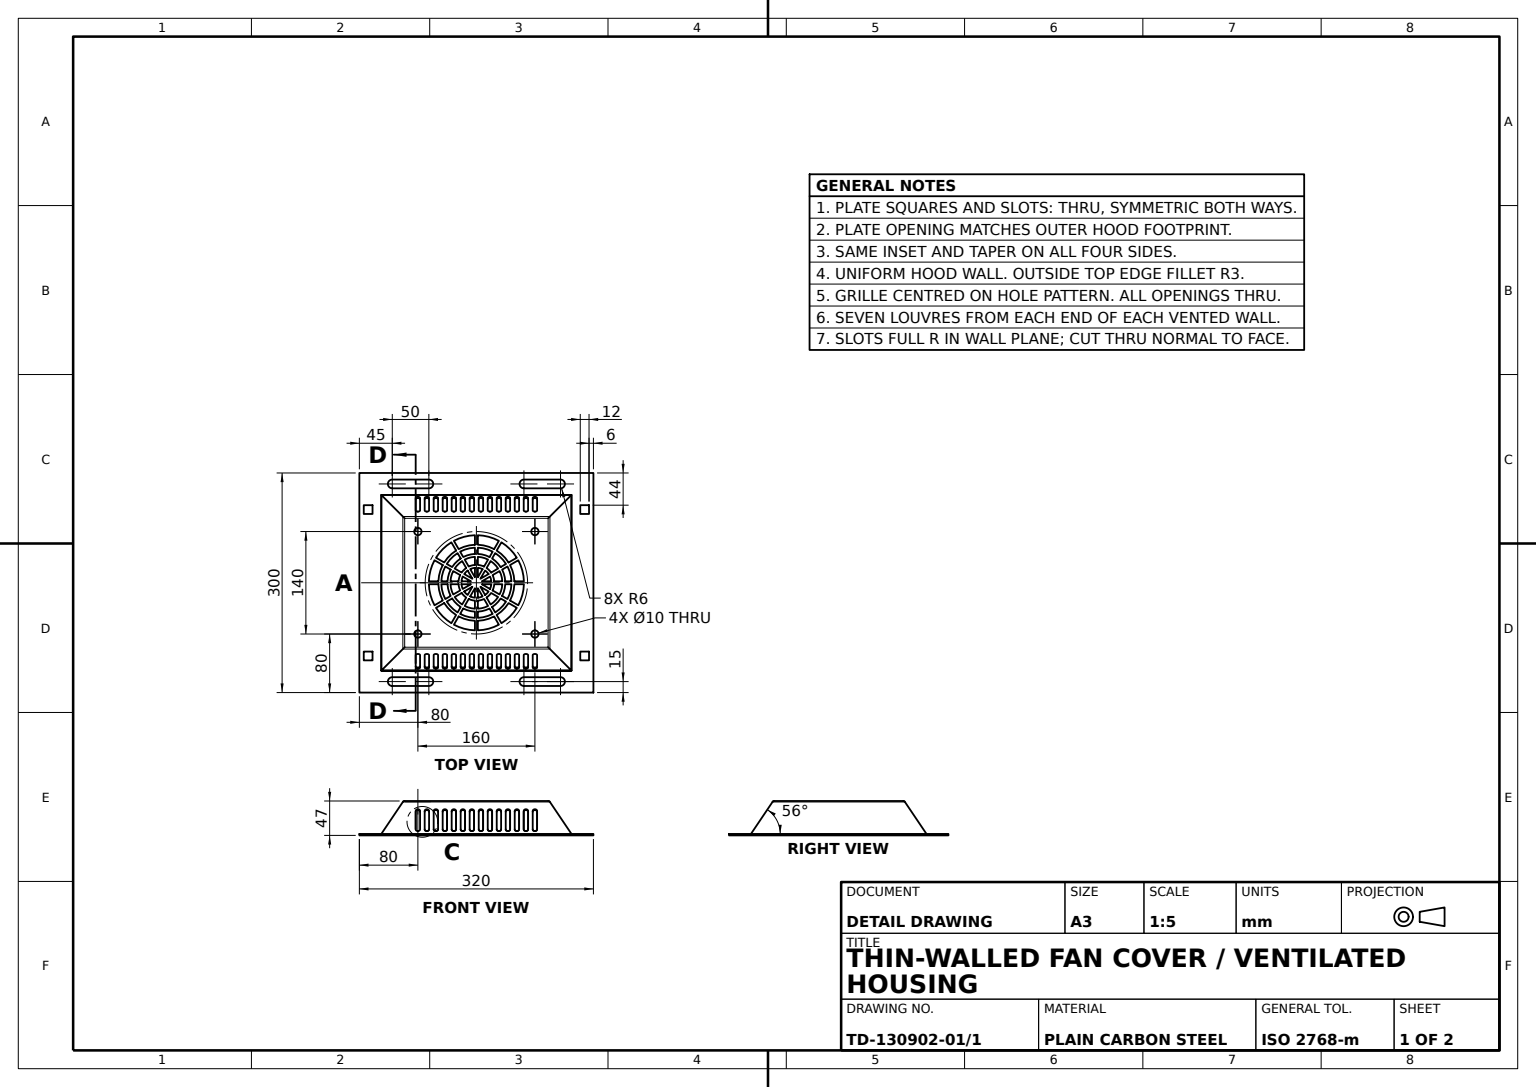
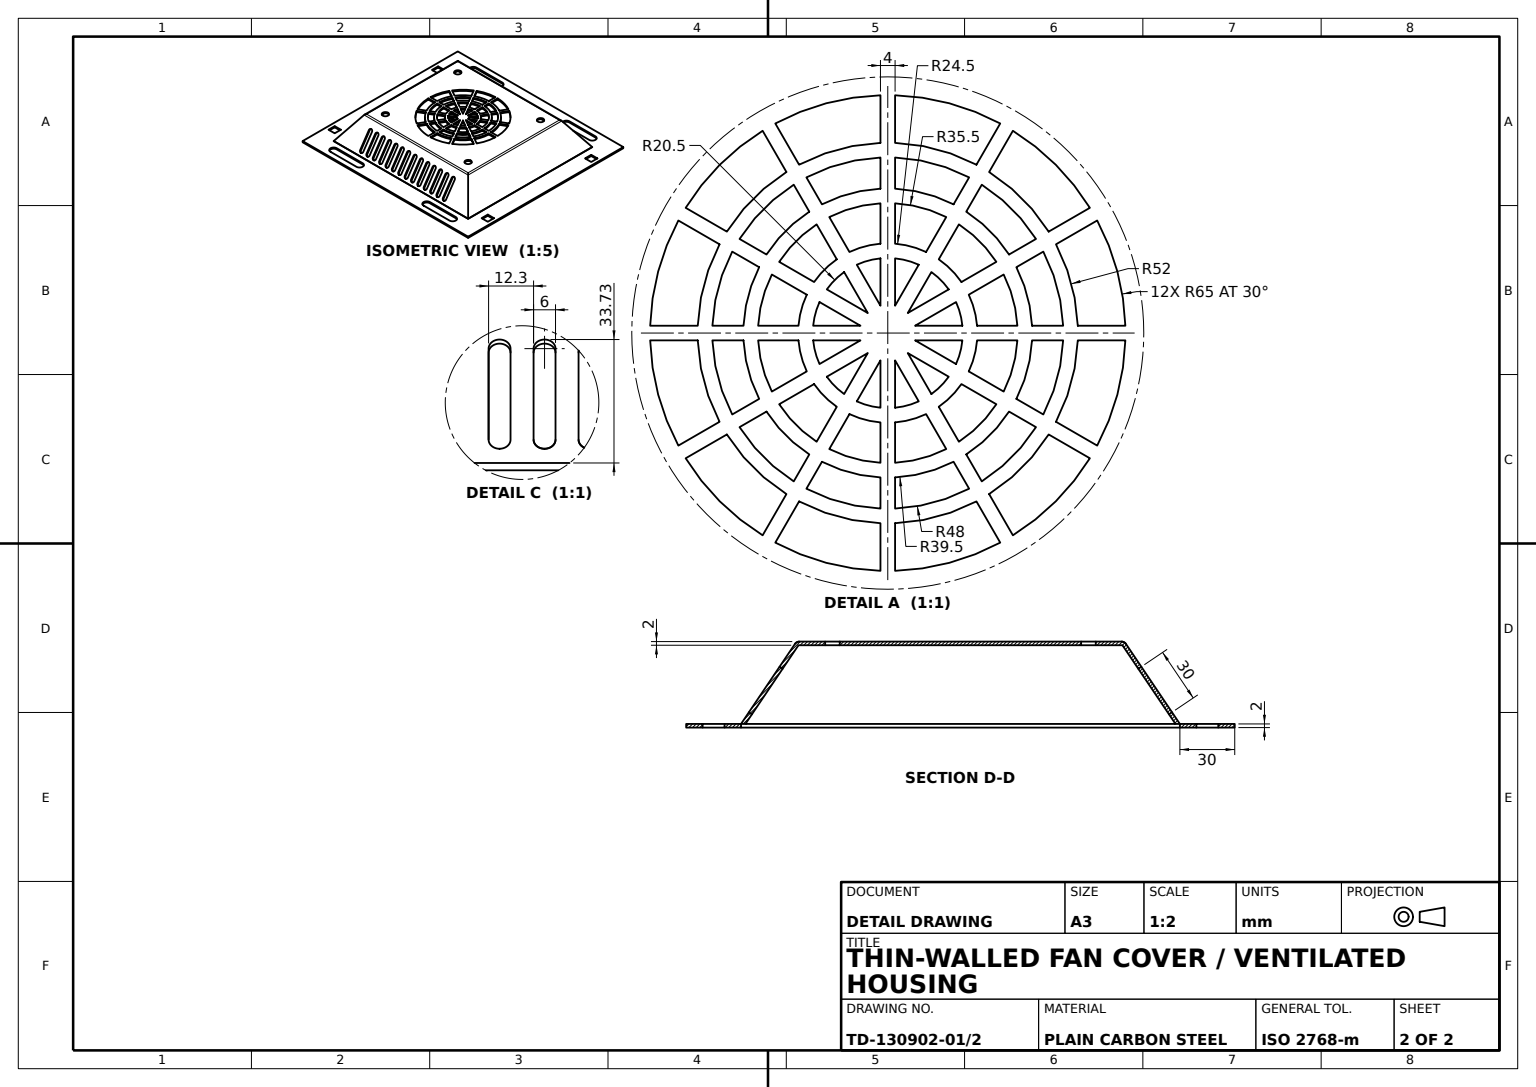
from build123d import *

# Parameters (mm, degrees)
BASE_PLATE_SKETCH_W                  = 320
BASE_PLATE_SKETCH_H                  = 300
BASE_PLATE_320X300X2_DEPTH           = 2
HOOD_FOOTPRINT_SKETCH_W              = 260
HOOD_FOOTPRINT_SKETCH_H              = 240
TAPERED_HOOD_H45_DEPTH               = 45
TAPERED_HOOD_H45_TAPER               = 34
HOOD_OPENING_SKETCH_W                = 260
HOOD_OPENING_SKETCH_H                = 240
HOOD_UNDERSIDE_OPENING_DEPTH         = 2
HOOD_SHELL_2MM_T                     = -2
FAN_GRILLE_CUT_DEPTH                 = 2
HOOD_EDGE_FILLET_R3_R                = 3
LOUVRE_SLOTS_SIDE_A_DEPTH            = 2
LOUVRE_SLOTS_SIDE_B_DEPTH            = 2
PLATE_MOUNTING_SLOTS_SKETCH_W        = 12
PLATE_MOUNTING_SLOTS_SKETCH_H        = 12
PLATE_MOUNTING_SLOTS_AND_HOLES_DEPTH = 2
HOOD_TOP_HOLES_SKETCH_R              = 5
HOOD_TOP_FIXING_HOLES_DEPTH          = 2


with BuildPart() as part:
    # Base Plate Sketch → Base Plate 320x300x2 (new body)
    with BuildSketch(Plane(origin=(0, 0, 0), x_dir=(1, 0, 0), z_dir=(0, 1, 0))):
        Rectangle(BASE_PLATE_SKETCH_W, BASE_PLATE_SKETCH_H)
    extrude(amount=BASE_PLATE_320X300X2_DEPTH)

    # Hood Footprint Sketch → Tapered Hood H45 (add)
    with BuildSketch(Plane(origin=(0, 2, 0), x_dir=(1, 0, 0), z_dir=(0, 1, 0))):
        Rectangle(HOOD_FOOTPRINT_SKETCH_W, HOOD_FOOTPRINT_SKETCH_H)
    extrude(amount=TAPERED_HOOD_H45_DEPTH, taper=TAPERED_HOOD_H45_TAPER)

    # Hood Opening Sketch → Hood Underside Opening (cut)
    with BuildSketch(Plane.XZ):
        Rectangle(HOOD_OPENING_SKETCH_W, HOOD_OPENING_SKETCH_H)
    extrude(amount=-HOOD_UNDERSIDE_OPENING_DEPTH, mode=Mode.SUBTRACT)


with BuildPart() as hood_underside_opening_piece_1:
    # of the separate pieces the step leaves, piece 1, a body of its own (hood_underside_opening_pieces)
    add(part.part.solids().sort_by_distance((99.647116742, 47, 89.647116742))[0])

    # Hood Shell 2mm
    hood_shell_2mm_openings = [hood_underside_opening_piece_1.faces().sort_by_distance(p)[0] for p in [
        (0, 2, 0),
    ]]
    offset(amount=HOOD_SHELL_2MM_T, openings=hood_shell_2mm_openings, kind=Kind.INTERSECTION)

    # Fan Grille Sketch → Fan Grille Cut (cut)
    with BuildSketch(Plane(origin=(0, 47, 0), x_dir=(1, 0, 0), z_dir=(0, 1, 0))):
        with BuildLine():
            ThreePointArc((-27.712812921, 44), (-36.769552622, 36.769552622), (-44, 27.712812921))
            Line((-44, 27.712812921), (-55.264998001, 34.216662549))
            ThreePointArc((-55.264998001, 34.216662549), (-45.961940777, 45.961940777), (-34.216662549, 55.264998001))
            Line((-34.216662549, 55.264998001), (-27.712812921, 44))
        make_face()
        with BuildLine():
            Line((-30.752560934, 57.264998001), (-24.248711306, 46))
            ThreePointArc((-24.248711306, 46), (-13.458590345, 50.228142967), (-2, 51.961524227))
            Line((-2, 51.961524227), (-2, 64.969223483))
            ThreePointArc((-2, 64.969223483), (-16.823237932, 62.785178709), (-30.752560934, 57.264998001))
        make_face()
        with BuildLine():
            ThreePointArc((30.752560934, 57.264998001), (16.823237932, 62.785178709), (2, 64.969223483))
            Line((2, 64.969223483), (2, 51.961524227))
            ThreePointArc((2, 51.961524227), (13.458590345, 50.228142967), (24.248711306, 46))
            Line((24.248711306, 46), (30.752560934, 57.264998001))
        make_face()
        with BuildLine():
            ThreePointArc((44, 27.712812921), (36.769552622, 36.769552622), (27.712812921, 44))
            Line((27.712812921, 44), (34.216662549, 55.264998001))
            ThreePointArc((34.216662549, 55.264998001), (45.961940777, 45.961940777), (55.264998001, 34.216662549))
            Line((55.264998001, 34.216662549), (44, 27.712812921))
        make_face()
        with BuildLine():
            ThreePointArc((51.961524227, 2), (50.228142967, 13.458590345), (46, 24.248711306))
            Line((46, 24.248711306), (57.264998001, 30.752560934))
            ThreePointArc((57.264998001, 30.752560934), (62.785178709, 16.823237932), (64.969223483, 2))
            Line((64.969223483, 2), (51.961524227, 2))
        make_face()
        with BuildLine():
            ThreePointArc((46, -24.248711306), (50.228142967, -13.458590345), (51.961524227, -2))
            Line((51.961524227, -2), (64.969223483, -2))
            ThreePointArc((64.969223483, -2), (62.785178709, -16.823237932), (57.264998001, -30.752560934))
            Line((57.264998001, -30.752560934), (46, -24.248711306))
        make_face()
        with BuildLine():
            ThreePointArc((27.712812921, -44), (36.769552622, -36.769552622), (44, -27.712812921))
            Line((44, -27.712812921), (55.264998001, -34.216662549))
            ThreePointArc((55.264998001, -34.216662549), (45.961940777, -45.961940777), (34.216662549, -55.264998001))
            Line((34.216662549, -55.264998001), (27.712812921, -44))
        make_face()
        with BuildLine():
            ThreePointArc((2, -51.961524227), (13.458590345, -50.228142967), (24.248711306, -46))
            Line((24.248711306, -46), (30.752560934, -57.264998001))
            ThreePointArc((30.752560934, -57.264998001), (16.823237932, -62.785178709), (2, -64.969223483))
            Line((2, -64.969223483), (2, -51.961524227))
        make_face()
        with BuildLine():
            ThreePointArc((-24.248711306, -46), (-13.458590345, -50.228142967), (-2, -51.961524227))
            Line((-2, -51.961524227), (-2, -64.969223483))
            ThreePointArc((-2, -64.969223483), (-16.823237932, -62.785178709), (-30.752560934, -57.264998001))
            Line((-30.752560934, -57.264998001), (-24.248711306, -46))
        make_face()
        with BuildLine():
            ThreePointArc((-44, -27.712812921), (-36.769552622, -36.769552622), (-27.712812921, -44))
            Line((-27.712812921, -44), (-34.216662549, -55.264998001))
            ThreePointArc((-34.216662549, -55.264998001), (-45.961940777, -45.961940777), (-55.264998001, -34.216662549))
            Line((-55.264998001, -34.216662549), (-44, -27.712812921))
        make_face()
        with BuildLine():
            ThreePointArc((-51.961524227, -2), (-50.228142967, -13.458590345), (-46, -24.248711306))
            Line((-46, -24.248711306), (-57.264998001, -30.752560934))
            ThreePointArc((-57.264998001, -30.752560934), (-62.785178709, -16.823237932), (-64.969223483, -2))
            Line((-64.969223483, -2), (-51.961524227, -2))
        make_face()
        with BuildLine():
            ThreePointArc((-46, 24.248711306), (-50.228142967, 13.458590345), (-51.961524227, 2))
            Line((-51.961524227, 2), (-64.969223483, 2))
            ThreePointArc((-64.969223483, 2), (-62.785178709, 16.823237932), (-57.264998001, 30.752560934))
            Line((-57.264998001, 30.752560934), (-46, 24.248711306))
        make_face()
        with BuildLine():
            ThreePointArc((-35.164125922, 17.99261649), (-38.154070138, 10.223352282), (-39.449334595, 2))
            Line((-39.449334595, 2), (-47.958315233, 2))
            ThreePointArc((-47.958315233, 2), (-46.364439662, 12.423314165), (-42.533119315, 22.247106809))
            Line((-42.533119315, 22.247106809), (-35.164125922, 17.99261649))
        make_face()
        with BuildLine():
            ThreePointArc((-21.456718105, 33.164125922), (-27.930717857, 27.930717857), (-33.164125922, 21.456718105))
            Line((-33.164125922, 21.456718105), (-40.533119315, 25.711208424))
            ThreePointArc((-40.533119315, 25.711208424), (-33.941125497, 33.941125497), (-25.711208424, 40.533119315))
            Line((-25.711208424, 40.533119315), (-21.456718105, 33.164125922))
        make_face()
        with BuildLine():
            ThreePointArc((-2, 39.449334595), (-10.223352282, 38.154070138), (-17.99261649, 35.164125922))
            Line((-17.99261649, 35.164125922), (-22.247106809, 42.533119315))
            ThreePointArc((-22.247106809, 42.533119315), (-12.423314165, 46.364439662), (-2, 47.958315233))
            Line((-2, 47.958315233), (-2, 39.449334595))
        make_face()
        with BuildLine():
            ThreePointArc((17.99261649, 35.164125922), (10.223352282, 38.154070138), (2, 39.449334595))
            Line((2, 39.449334595), (2, 47.958315233))
            ThreePointArc((2, 47.958315233), (12.423314165, 46.364439662), (22.247106809, 42.533119315))
            Line((22.247106809, 42.533119315), (17.99261649, 35.164125922))
        make_face()
        with BuildLine():
            ThreePointArc((33.164125922, 21.456718105), (27.930717857, 27.930717857), (21.456718105, 33.164125922))
            Line((21.456718105, 33.164125922), (25.711208424, 40.533119315))
            ThreePointArc((25.711208424, 40.533119315), (33.941125497, 33.941125497), (40.533119315, 25.711208424))
            Line((40.533119315, 25.711208424), (33.164125922, 21.456718105))
        make_face()
        with BuildLine():
            ThreePointArc((39.449334595, 2), (38.154070138, 10.223352282), (35.164125922, 17.99261649))
            Line((35.164125922, 17.99261649), (42.533119315, 22.247106809))
            ThreePointArc((42.533119315, 22.247106809), (46.364439662, 12.423314165), (47.958315233, 2))
            Line((47.958315233, 2), (39.449334595, 2))
        make_face()
        with BuildLine():
            ThreePointArc((35.164125922, -17.99261649), (38.154070138, -10.223352282), (39.449334595, -2))
            Line((39.449334595, -2), (47.958315233, -2))
            ThreePointArc((47.958315233, -2), (46.364439662, -12.423314165), (42.533119315, -22.247106809))
            Line((42.533119315, -22.247106809), (35.164125922, -17.99261649))
        make_face()
        with BuildLine():
            ThreePointArc((21.456718105, -33.164125922), (27.930717857, -27.930717857), (33.164125922, -21.456718105))
            Line((33.164125922, -21.456718105), (40.533119315, -25.711208424))
            ThreePointArc((40.533119315, -25.711208424), (33.941125497, -33.941125497), (25.711208424, -40.533119315))
            Line((25.711208424, -40.533119315), (21.456718105, -33.164125922))
        make_face()
        with BuildLine():
            ThreePointArc((2, -39.449334595), (10.223352282, -38.154070138), (17.99261649, -35.164125922))
            Line((17.99261649, -35.164125922), (22.247106809, -42.533119315))
            ThreePointArc((22.247106809, -42.533119315), (12.423314165, -46.364439662), (2, -47.958315233))
            Line((2, -47.958315233), (2, -39.449334595))
        make_face()
        with BuildLine():
            ThreePointArc((-17.99261649, -35.164125922), (-10.223352282, -38.154070138), (-2, -39.449334595))
            Line((-2, -39.449334595), (-2, -47.958315233))
            ThreePointArc((-2, -47.958315233), (-12.423314165, -46.364439662), (-22.247106809, -42.533119315))
            Line((-22.247106809, -42.533119315), (-17.99261649, -35.164125922))
        make_face()
        with BuildLine():
            ThreePointArc((-33.164125922, -21.456718105), (-27.930717857, -27.930717857), (-21.456718105, -33.164125922))
            Line((-21.456718105, -33.164125922), (-25.711208424, -40.533119315))
            ThreePointArc((-25.711208424, -40.533119315), (-33.941125497, -33.941125497), (-40.533119315, -25.711208424))
            Line((-40.533119315, -25.711208424), (-33.164125922, -21.456718105))
        make_face()
        with BuildLine():
            ThreePointArc((-39.449334595, -2), (-38.154070138, -10.223352282), (-35.164125922, -17.99261649))
            Line((-35.164125922, -17.99261649), (-42.533119315, -22.247106809))
            ThreePointArc((-42.533119315, -22.247106809), (-46.364439662, -12.423314165), (-47.958315233, -2))
            Line((-47.958315233, -2), (-39.449334595, -2))
        make_face()
        with BuildLine():
            ThreePointArc((-10.47706464, -22.14680827), (-6.341066605, -23.665182744), (-2, -24.418230894))
            Line((-2, -24.418230894), (-2, -35.443617197))
            ThreePointArc((-2, -35.443617197), (-9.188076101, -34.290366833), (-15.989757791, -31.695072895))
            Line((-15.989757791, -31.695072895), (-10.47706464, -22.14680827))
        make_face()
        with BuildLine():
            ThreePointArc((-20.14680827, -13.941166255), (-17.324116139, -17.324116139), (-13.941166255, -20.14680827))
            Line((-13.941166255, -20.14680827), (-19.453859406, -29.695072895))
            ThreePointArc((-19.453859406, -29.695072895), (-25.102290732, -25.102290732), (-29.695072895, -19.453859406))
            Line((-29.695072895, -19.453859406), (-20.14680827, -13.941166255))
        make_face()
        with BuildLine():
            ThreePointArc((-24.418230894, -2), (-23.665182744, -6.341066605), (-22.14680827, -10.47706464))
            Line((-22.14680827, -10.47706464), (-31.695072895, -15.989757791))
            ThreePointArc((-31.695072895, -15.989757791), (-34.290366833, -9.188076101), (-35.443617197, -2))
            Line((-35.443617197, -2), (-24.418230894, -2))
        make_face()
        with BuildLine():
            ThreePointArc((-22.14680827, 10.47706464), (-23.665182744, 6.341066605), (-24.418230894, 2))
            Line((-24.418230894, 2), (-35.443617197, 2))
            ThreePointArc((-35.443617197, 2), (-34.290366833, 9.188076101), (-31.695072895, 15.989757791))
            Line((-31.695072895, 15.989757791), (-22.14680827, 10.47706464))
        make_face()
        with BuildLine():
            ThreePointArc((-13.941166255, 20.14680827), (-17.324116139, 17.324116139), (-20.14680827, 13.941166255))
            Line((-20.14680827, 13.941166255), (-29.695072895, 19.453859406))
            ThreePointArc((-29.695072895, 19.453859406), (-25.102290732, 25.102290732), (-19.453859406, 29.695072895))
            Line((-19.453859406, 29.695072895), (-13.941166255, 20.14680827))
        make_face()
        with BuildLine():
            ThreePointArc((-2, 24.418230894), (-6.341066605, 23.665182744), (-10.47706464, 22.14680827))
            Line((-10.47706464, 22.14680827), (-15.989757791, 31.695072895))
            ThreePointArc((-15.989757791, 31.695072895), (-9.188076101, 34.290366833), (-2, 35.443617197))
            Line((-2, 35.443617197), (-2, 24.418230894))
        make_face()
        with BuildLine():
            ThreePointArc((10.47706464, 22.14680827), (6.341066605, 23.665182744), (2, 24.418230894))
            Line((2, 24.418230894), (2, 35.443617197))
            ThreePointArc((2, 35.443617197), (9.188076101, 34.290366833), (15.989757791, 31.695072895))
            Line((15.989757791, 31.695072895), (10.47706464, 22.14680827))
        make_face()
        with BuildLine():
            ThreePointArc((20.14680827, 13.941166255), (17.324116139, 17.324116139), (13.941166255, 20.14680827))
            Line((13.941166255, 20.14680827), (19.453859406, 29.695072895))
            ThreePointArc((19.453859406, 29.695072895), (25.102290732, 25.102290732), (29.695072895, 19.453859406))
            Line((29.695072895, 19.453859406), (20.14680827, 13.941166255))
        make_face()
        with BuildLine():
            ThreePointArc((24.418230894, 2), (23.665182744, 6.341066605), (22.14680827, 10.47706464))
            Line((22.14680827, 10.47706464), (31.695072895, 15.989757791))
            ThreePointArc((31.695072895, 15.989757791), (34.290366833, 9.188076101), (35.443617197, 2))
            Line((35.443617197, 2), (24.418230894, 2))
        make_face()
        with BuildLine():
            ThreePointArc((22.14680827, -10.47706464), (23.665182744, -6.341066605), (24.418230894, -2))
            Line((24.418230894, -2), (35.443617197, -2))
            ThreePointArc((35.443617197, -2), (34.290366833, -9.188076101), (31.695072895, -15.989757791))
            Line((31.695072895, -15.989757791), (22.14680827, -10.47706464))
        make_face()
        with BuildLine():
            ThreePointArc((13.941166255, -20.14680827), (17.324116139, -17.324116139), (20.14680827, -13.941166255))
            Line((20.14680827, -13.941166255), (29.695072895, -19.453859406))
            ThreePointArc((29.695072895, -19.453859406), (25.102290732, -25.102290732), (19.453859406, -29.695072895))
            Line((19.453859406, -29.695072895), (13.941166255, -20.14680827))
        make_face()
        with BuildLine():
            ThreePointArc((2, -24.418230894), (6.341066605, -23.665182744), (10.47706464, -22.14680827))
            Line((10.47706464, -22.14680827), (15.989757791, -31.695072895))
            ThreePointArc((15.989757791, -31.695072895), (9.188076101, -34.290366833), (2, -35.443617197))
            Line((2, -35.443617197), (2, -24.418230894))
        make_face()
        with BuildLine():
            Line((2, 7.464101615), (8.469052074, 18.668828484))
            ThreePointArc((8.469052074, 18.668828484), (5.305790425, 19.801479439), (2, 20.402205763))
            Line((2, 20.402205763), (2, 7.464101615))
        make_face()
        with BuildLine():
            Line((5.464101615, 5.464101615), (16.668828484, 11.933153689))
            ThreePointArc((16.668828484, 11.933153689), (14.495689014, 14.495689014), (11.933153689, 16.668828484))
            Line((11.933153689, 16.668828484), (5.464101615, 5.464101615))
        make_face()
        with BuildLine():
            Line((7.464101615, 2), (20.402205763, 2))
            ThreePointArc((20.402205763, 2), (19.801479439, 5.305790425), (18.668828484, 8.469052074))
            Line((18.668828484, 8.469052074), (7.464101615, 2))
        make_face()
        with BuildLine():
            Line((7.464101615, -2), (18.668828484, -8.469052074))
            ThreePointArc((18.668828484, -8.469052074), (19.801479439, -5.305790425), (20.402205763, -2))
            Line((20.402205763, -2), (7.464101615, -2))
        make_face()
        with BuildLine():
            Line((5.464101615, -5.464101615), (11.933153689, -16.668828484))
            ThreePointArc((11.933153689, -16.668828484), (14.495689014, -14.495689014), (16.668828484, -11.933153689))
            Line((16.668828484, -11.933153689), (5.464101615, -5.464101615))
        make_face()
        with BuildLine():
            Line((2, -20.402205763), (2, -7.464101615))
            Line((2, -7.464101615), (8.469052074, -18.668828484))
            ThreePointArc((8.469052074, -18.668828484), (5.305790425, -19.801479439), (2, -20.402205763))
        make_face()
        with BuildLine():
            Line((-2, -7.464101615), (-8.469052074, -18.668828484))
            ThreePointArc((-8.469052074, -18.668828484), (-5.305790425, -19.801479439), (-2, -20.402205763))
            Line((-2, -20.402205763), (-2, -7.464101615))
        make_face()
        with BuildLine():
            Line((-5.464101615, -5.464101615), (-16.668828484, -11.933153689))
            ThreePointArc((-16.668828484, -11.933153689), (-14.495689014, -14.495689014), (-11.933153689, -16.668828484))
            Line((-11.933153689, -16.668828484), (-5.464101615, -5.464101615))
        make_face()
        with BuildLine():
            Line((-20.402205763, -2), (-7.464101615, -2))
            Line((-7.464101615, -2), (-18.668828484, -8.469052074))
            ThreePointArc((-18.668828484, -8.469052074), (-19.801479439, -5.305790425), (-20.402205763, -2))
        make_face()
        with BuildLine():
            Line((-7.464101615, 2), (-18.668828484, 8.469052074))
            ThreePointArc((-18.668828484, 8.469052074), (-19.801479439, 5.305790425), (-20.402205763, 2))
            Line((-20.402205763, 2), (-7.464101615, 2))
        make_face()
        with BuildLine():
            Line((-5.464101615, 5.464101615), (-11.933153689, 16.668828484))
            ThreePointArc((-11.933153689, 16.668828484), (-14.495689014, 14.495689014), (-16.668828484, 11.933153689))
            Line((-16.668828484, 11.933153689), (-5.464101615, 5.464101615))
        make_face()
        with BuildLine():
            Line((-2, 7.464101615), (-2, 20.402205763))
            ThreePointArc((-2, 20.402205763), (-5.305790425, 19.801479439), (-8.469052074, 18.668828484))
            Line((-8.469052074, 18.668828484), (-2, 7.464101615))
        make_face()
    extrude(amount=-FAN_GRILLE_CUT_DEPTH, mode=Mode.SUBTRACT)

    # Hood Edge Fillet R3
    hood_edge_fillet_r3_edges = [hood_underside_opening_piece_1.edges().sort_by_distance(p)[0] for p in [
        (99.647116742, 47, 0),
        (0, 47, -89.647116742),
        (-99.647116742, 47, 0),
        (0, 47, 89.647116742),
    ]]
    fillet(hood_edge_fillet_r3_edges, radius=HOOD_EDGE_FILLET_R3_R)

    # Louvre Slots Side A Sketch → Louvre Slots Side A (cut)
    with BuildSketch(Plane(origin=(0, 56.256424681, 83.40357946), x_dir=(1, 0, 0), z_dir=(0, 0.5591929034707479, 0.829037572555041))):
        with BuildLine():
            Line((-77, -27.760393884), (-77, -57.760393884))
            ThreePointArc((-77, -57.760393884), (-80, -60.760393884), (-83, -57.760393884))
            Line((-83, -57.760393884), (-83, -27.760393884))
            ThreePointArc((-83, -27.760393884), (-80, -24.760393884), (-77, -27.760393884))
        make_face()
        with BuildLine():
            Line((83, -27.760393884), (83, -57.760393884))
            ThreePointArc((83, -57.760393884), (80, -60.760393884), (77, -57.760393884))
            Line((77, -57.760393884), (77, -27.760393884))
            ThreePointArc((77, -27.760393884), (80, -24.760393884), (83, -27.760393884))
        make_face()
        with BuildLine():
            Line((70.7, -27.760393884), (70.7, -57.760393884))
            ThreePointArc((70.7, -57.760393884), (67.7, -60.760393884), (64.7, -57.760393884))
            Line((64.7, -57.760393884), (64.7, -27.760393884))
            ThreePointArc((64.7, -27.760393884), (67.7, -24.760393884), (70.7, -27.760393884))
        make_face()
        with BuildLine():
            Line((58.4, -27.760393884), (58.4, -57.760393884))
            ThreePointArc((58.4, -57.760393884), (55.4, -60.760393884), (52.4, -57.760393884))
            Line((52.4, -57.760393884), (52.4, -27.760393884))
            ThreePointArc((52.4, -27.760393884), (55.4, -24.760393884), (58.4, -27.760393884))
        make_face()
        with BuildLine():
            Line((46.1, -27.760393884), (46.1, -57.760393884))
            ThreePointArc((46.1, -57.760393884), (43.1, -60.760393884), (40.1, -57.760393884))
            Line((40.1, -57.760393884), (40.1, -27.760393884))
            ThreePointArc((40.1, -27.760393884), (43.1, -24.760393884), (46.1, -27.760393884))
        make_face()
        with BuildLine():
            Line((33.8, -27.760393884), (33.8, -57.760393884))
            ThreePointArc((33.8, -57.760393884), (30.8, -60.760393884), (27.8, -57.760393884))
            Line((27.8, -57.760393884), (27.8, -27.760393884))
            ThreePointArc((27.8, -27.760393884), (30.8, -24.760393884), (33.8, -27.760393884))
        make_face()
        with BuildLine():
            Line((21.5, -27.760393884), (21.5, -57.760393884))
            ThreePointArc((21.5, -57.760393884), (18.5, -60.760393884), (15.5, -57.760393884))
            Line((15.5, -57.760393884), (15.5, -27.760393884))
            ThreePointArc((15.5, -27.760393884), (18.5, -24.760393884), (21.5, -27.760393884))
        make_face()
        with BuildLine():
            Line((9.2, -27.760393884), (9.2, -57.760393884))
            ThreePointArc((9.2, -57.760393884), (6.2, -60.760393884), (3.2, -57.760393884))
            Line((3.2, -57.760393884), (3.2, -27.760393884))
            ThreePointArc((3.2, -27.760393884), (6.2, -24.760393884), (9.2, -27.760393884))
        make_face()
        with BuildLine():
            Line((-64.7, -27.760393884), (-64.7, -57.760393884))
            ThreePointArc((-64.7, -57.760393884), (-67.7, -60.760393884), (-70.7, -57.760393884))
            Line((-70.7, -57.760393884), (-70.7, -27.760393884))
            ThreePointArc((-70.7, -27.760393884), (-67.7, -24.760393884), (-64.7, -27.760393884))
        make_face()
        with BuildLine():
            Line((-52.4, -27.760393884), (-52.4, -57.760393884))
            ThreePointArc((-52.4, -57.760393884), (-55.4, -60.760393884), (-58.4, -57.760393884))
            Line((-58.4, -57.760393884), (-58.4, -27.760393884))
            ThreePointArc((-58.4, -27.760393884), (-55.4, -24.760393884), (-52.4, -27.760393884))
        make_face()
        with BuildLine():
            Line((-40.1, -27.760393884), (-40.1, -57.760393884))
            ThreePointArc((-40.1, -57.760393884), (-43.1, -60.760393884), (-46.1, -57.760393884))
            Line((-46.1, -57.760393884), (-46.1, -27.760393884))
            ThreePointArc((-46.1, -27.760393884), (-43.1, -24.760393884), (-40.1, -27.760393884))
        make_face()
        with BuildLine():
            Line((-27.8, -27.760393884), (-27.8, -57.760393884))
            ThreePointArc((-27.8, -57.760393884), (-30.8, -60.760393884), (-33.8, -57.760393884))
            Line((-33.8, -57.760393884), (-33.8, -27.760393884))
            ThreePointArc((-33.8, -27.760393884), (-30.8, -24.760393884), (-27.8, -27.760393884))
        make_face()
        with BuildLine():
            Line((-15.5, -27.760393884), (-15.5, -57.760393884))
            ThreePointArc((-15.5, -57.760393884), (-18.5, -60.760393884), (-21.5, -57.760393884))
            Line((-21.5, -57.760393884), (-21.5, -27.760393884))
            ThreePointArc((-21.5, -27.760393884), (-18.5, -24.760393884), (-15.5, -27.760393884))
        make_face()
        with BuildLine():
            Line((-3.2, -27.760393884), (-3.2, -57.760393884))
            ThreePointArc((-3.2, -57.760393884), (-6.2, -60.760393884), (-9.2, -57.760393884))
            Line((-9.2, -57.760393884), (-9.2, -27.760393884))
            ThreePointArc((-9.2, -27.760393884), (-6.2, -24.760393884), (-3.2, -27.760393884))
        make_face()
    extrude(amount=-LOUVRE_SLOTS_SIDE_A_DEPTH, mode=Mode.SUBTRACT)

    # Louvre Slots Side B Sketch → Louvre Slots Side B (cut)
    with BuildSketch(Plane(origin=(0, 56.256424681, -83.40357946), x_dir=(-1, 0, 0), z_dir=(0, 0.5591929034707479, -0.829037572555041))):
        with BuildLine():
            Line((-77, -27.760393884), (-77, -57.760393884))
            ThreePointArc((-77, -57.760393884), (-80, -60.760393884), (-83, -57.760393884))
            Line((-83, -57.760393884), (-83, -27.760393884))
            ThreePointArc((-83, -27.760393884), (-80, -24.760393884), (-77, -27.760393884))
        make_face()
        with BuildLine():
            Line((83, -27.760393884), (83, -57.760393884))
            ThreePointArc((83, -57.760393884), (80, -60.760393884), (77, -57.760393884))
            Line((77, -57.760393884), (77, -27.760393884))
            ThreePointArc((77, -27.760393884), (80, -24.760393884), (83, -27.760393884))
        make_face()
        with BuildLine():
            Line((70.7, -27.760393884), (70.7, -57.760393884))
            ThreePointArc((70.7, -57.760393884), (67.7, -60.760393884), (64.7, -57.760393884))
            Line((64.7, -57.760393884), (64.7, -27.760393884))
            ThreePointArc((64.7, -27.760393884), (67.7, -24.760393884), (70.7, -27.760393884))
        make_face()
        with BuildLine():
            Line((58.4, -27.760393884), (58.4, -57.760393884))
            ThreePointArc((58.4, -57.760393884), (55.4, -60.760393884), (52.4, -57.760393884))
            Line((52.4, -57.760393884), (52.4, -27.760393884))
            ThreePointArc((52.4, -27.760393884), (55.4, -24.760393884), (58.4, -27.760393884))
        make_face()
        with BuildLine():
            Line((46.1, -27.760393884), (46.1, -57.760393884))
            ThreePointArc((46.1, -57.760393884), (43.1, -60.760393884), (40.1, -57.760393884))
            Line((40.1, -57.760393884), (40.1, -27.760393884))
            ThreePointArc((40.1, -27.760393884), (43.1, -24.760393884), (46.1, -27.760393884))
        make_face()
        with BuildLine():
            Line((33.8, -27.760393884), (33.8, -57.760393884))
            ThreePointArc((33.8, -57.760393884), (30.8, -60.760393884), (27.8, -57.760393884))
            Line((27.8, -57.760393884), (27.8, -27.760393884))
            ThreePointArc((27.8, -27.760393884), (30.8, -24.760393884), (33.8, -27.760393884))
        make_face()
        with BuildLine():
            Line((21.5, -27.760393884), (21.5, -57.760393884))
            ThreePointArc((21.5, -57.760393884), (18.5, -60.760393884), (15.5, -57.760393884))
            Line((15.5, -57.760393884), (15.5, -27.760393884))
            ThreePointArc((15.5, -27.760393884), (18.5, -24.760393884), (21.5, -27.760393884))
        make_face()
        with BuildLine():
            Line((9.2, -27.760393884), (9.2, -57.760393884))
            ThreePointArc((9.2, -57.760393884), (6.2, -60.760393884), (3.2, -57.760393884))
            Line((3.2, -57.760393884), (3.2, -27.760393884))
            ThreePointArc((3.2, -27.760393884), (6.2, -24.760393884), (9.2, -27.760393884))
        make_face()
        with BuildLine():
            Line((-64.7, -27.760393884), (-64.7, -57.760393884))
            ThreePointArc((-64.7, -57.760393884), (-67.7, -60.760393884), (-70.7, -57.760393884))
            Line((-70.7, -57.760393884), (-70.7, -27.760393884))
            ThreePointArc((-70.7, -27.760393884), (-67.7, -24.760393884), (-64.7, -27.760393884))
        make_face()
        with BuildLine():
            Line((-52.4, -27.760393884), (-52.4, -57.760393884))
            ThreePointArc((-52.4, -57.760393884), (-55.4, -60.760393884), (-58.4, -57.760393884))
            Line((-58.4, -57.760393884), (-58.4, -27.760393884))
            ThreePointArc((-58.4, -27.760393884), (-55.4, -24.760393884), (-52.4, -27.760393884))
        make_face()
        with BuildLine():
            Line((-40.1, -27.760393884), (-40.1, -57.760393884))
            ThreePointArc((-40.1, -57.760393884), (-43.1, -60.760393884), (-46.1, -57.760393884))
            Line((-46.1, -57.760393884), (-46.1, -27.760393884))
            ThreePointArc((-46.1, -27.760393884), (-43.1, -24.760393884), (-40.1, -27.760393884))
        make_face()
        with BuildLine():
            Line((-27.8, -27.760393884), (-27.8, -57.760393884))
            ThreePointArc((-27.8, -57.760393884), (-30.8, -60.760393884), (-33.8, -57.760393884))
            Line((-33.8, -57.760393884), (-33.8, -27.760393884))
            ThreePointArc((-33.8, -27.760393884), (-30.8, -24.760393884), (-27.8, -27.760393884))
        make_face()
        with BuildLine():
            Line((-15.5, -27.760393884), (-15.5, -57.760393884))
            ThreePointArc((-15.5, -57.760393884), (-18.5, -60.760393884), (-21.5, -57.760393884))
            Line((-21.5, -57.760393884), (-21.5, -27.760393884))
            ThreePointArc((-21.5, -27.760393884), (-18.5, -24.760393884), (-15.5, -27.760393884))
        make_face()
        with BuildLine():
            Line((-3.2, -27.760393884), (-3.2, -57.760393884))
            ThreePointArc((-3.2, -57.760393884), (-6.2, -60.760393884), (-9.2, -57.760393884))
            Line((-9.2, -57.760393884), (-9.2, -27.760393884))
            ThreePointArc((-9.2, -27.760393884), (-6.2, -24.760393884), (-3.2, -27.760393884))
        make_face()
    extrude(amount=-LOUVRE_SLOTS_SIDE_B_DEPTH, mode=Mode.SUBTRACT)

    # Hood Top Holes Sketch → Hood Top Fixing Holes (cut)
    with BuildSketch(Plane(origin=(0, 47, 0), x_dir=(1, 0, 0), z_dir=(0, 1, 0))):
        with Locations(Location((-80, 70, 0), (0, 0, 270))):
            Circle(HOOD_TOP_HOLES_SKETCH_R)
        with Locations(Location((80, 70, 0), (0, 0, 270))):
            Circle(HOOD_TOP_HOLES_SKETCH_R)
        with Locations(Location((80, -70, 0), (0, 0, 270))):
            Circle(HOOD_TOP_HOLES_SKETCH_R)
        with Locations(Location((-80, -70, 0), (0, 0, 270))):
            Circle(HOOD_TOP_HOLES_SKETCH_R)
    extrude(amount=-HOOD_TOP_FIXING_HOLES_DEPTH, mode=Mode.SUBTRACT)


with BuildPart() as hood_underside_opening_piece_2:
    # of the separate pieces the step leaves, piece 2, a body of its own (hood_underside_opening_pieces)
    add(part.part.solids().sort_by_distance((-160, 0, 150))[0])

    # Plate Mounting Slots Sketch → Plate Mounting Slots and Holes (cut)
    with BuildSketch(Plane(origin=(0, 2, 0), x_dir=(1, 0, 0), z_dir=(0, 1, 0))):
        with BuildLine():
            Line((-115, -129), (-65, -129))
            ThreePointArc((-65, -129), (-59, -135), (-65, -141))
            Line((-65, -141), (-115, -141))
            ThreePointArc((-115, -141), (-121, -135), (-115, -129))
        make_face()
        with BuildLine():
            Line((65, -129), (115, -129))
            ThreePointArc((115, -129), (121, -135), (115, -141))
            Line((115, -141), (65, -141))
            ThreePointArc((65, -141), (59, -135), (65, -129))
        make_face()
        with BuildLine():
            Line((-115, 141), (-65, 141))
            ThreePointArc((-65, 141), (-59, 135), (-65, 129))
            Line((-65, 129), (-115, 129))
            ThreePointArc((-115, 129), (-121, 135), (-115, 141))
        make_face()
        with BuildLine():
            Line((65, 141), (115, 141))
            ThreePointArc((115, 141), (121, 135), (115, 129))
            Line((115, 129), (65, 129))
            ThreePointArc((65, 129), (59, 135), (65, 141))
        make_face()
        with Locations((148, 100)):
            Rectangle(PLATE_MOUNTING_SLOTS_SKETCH_W, PLATE_MOUNTING_SLOTS_SKETCH_H)
        with Locations((148, -100)):
            Rectangle(PLATE_MOUNTING_SLOTS_SKETCH_W, PLATE_MOUNTING_SLOTS_SKETCH_H)
        with Locations((-148, -100)):
            Rectangle(PLATE_MOUNTING_SLOTS_SKETCH_W, PLATE_MOUNTING_SLOTS_SKETCH_H)
        with Locations((-148, 100)):
            Rectangle(PLATE_MOUNTING_SLOTS_SKETCH_W, PLATE_MOUNTING_SLOTS_SKETCH_H)
    extrude(amount=-PLATE_MOUNTING_SLOTS_AND_HOLES_DEPTH, mode=Mode.SUBTRACT)


solid = Compound([hood_underside_opening_piece_1.part, hood_underside_opening_piece_2.part])
